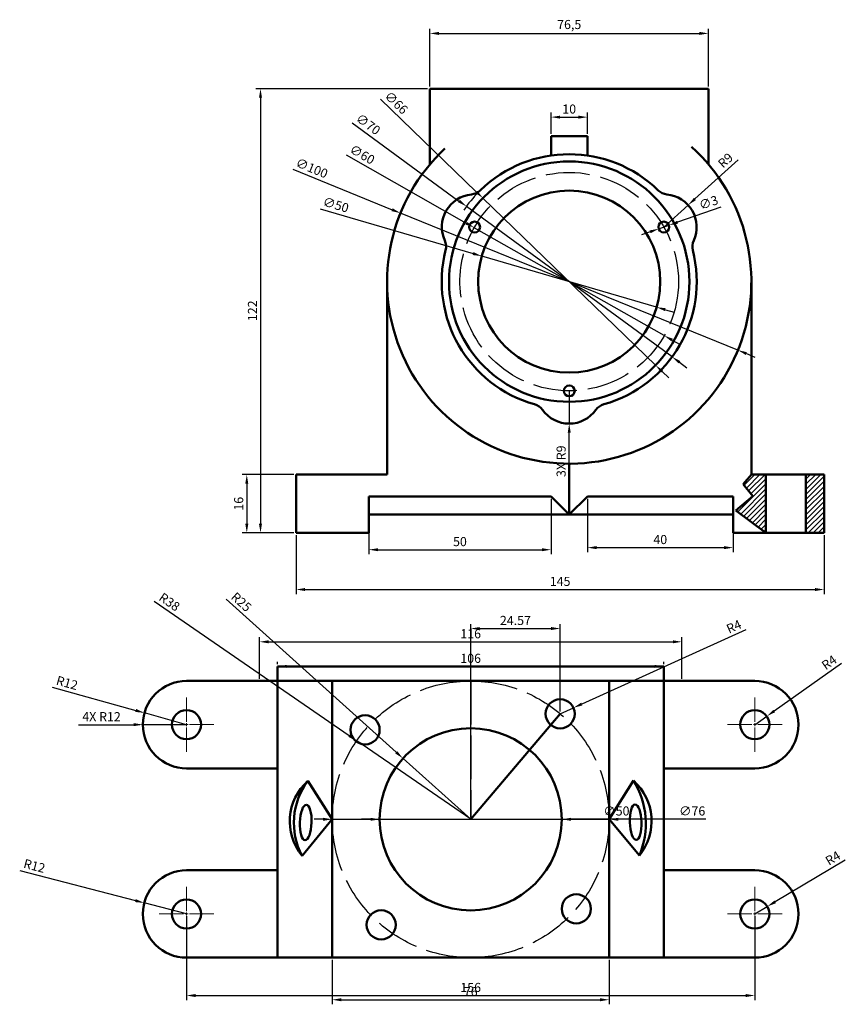
# Model space of a CAD drawing. Units: millimetres. Extents: x 1140 to 1880, y 1480 to 1815.
# Tile 1 of 3: x 1140 to 1366, y 1537 to 1807. Entities that reach past the tile are written whole.
import ezdxf

# ---------------------------------------------------------------- set-up
doc = ezdxf.new("R2010")
doc.units = ezdxf.units.MM
doc.linetypes.add('ACAD_ISO02W100', pattern=[15, 12, -3])
doc.linetypes.add('CENTER2', pattern=[28.575, 19.05, -3.175, 3.175, -3.175])
for name, color, linetype, lineweight in [('M-CNTR', 1, 'CENTER2', 18), ('M-DIMS', 2, 'Continuous', 25), ('M-HATC', 8, 'Continuous', 18), ('M-HIDN', 6, 'ACAD_ISO02W100', 25), ('M-OUTL', 7, 'Continuous', 50)]:
    doc.layers.add(name, color=color, linetype=linetype, lineweight=lineweight)
doc.styles.get("Standard").update_dxf_attribs({"font": 'arial.ttf'})
doc.dimstyles.new('ISO-25', dxfattribs={"dimtxt": 2.5, "dimasz": 2.5, "dimexe": 1.25, "dimexo": 0.625, "dimtad": 1, "dimtxsty": 'Standard', "dimcen": 2.5, "dimadec": 0, "dimazin": 0, "dimtfac": 1, "dimtmove": 0, "dimatfit": 3, "dimfxl": 1, "dimarcsym": 0})

# ---------------------------------------------------------------- blocks, each defined once
blk = doc.blocks.new('*U1')
blk.add_circle((0, 0), 1.5)
blk = doc.blocks.new('*U2')
at = {"layer": 'M-OUTL', "color": 0, "linetype": 'ByBlock', "lineweight": -2, "transparency": 16777216}
for p, rotation in [((1264.48, 1750.45), 240), ((1316.44, 1750.45), 119.9999999999999)]:
    blk.add_blockref('*U1', p, dxfattribs=dict(at, rotation=rotation))
blk.add_blockref('*U1', (1290.46, 1705.45), dxfattribs=at)
blk = doc.blocks.new('*U3')
at = {"layer": 'M-CNTR', "color": 0, "transparency": 16777216}
for p, q in [((0, 0.8), (0, 7.5)), ((-7.5, 0), (-0.8, 0)), ((0.8, 0), (7.5, 0)), ((0, -7.5), (0, -0.8))]:
    blk.add_line(p, q, dxfattribs=at)
at = {"layer": 'M-CNTR', "color": 0, "linetype": 'Continuous', "transparency": 16777216}
for p, q in [((-0.4, 0), (0.4, 0)), ((0, -0.4), (0, 0.4))]:
    blk.add_line(p, q, dxfattribs=at)
blk = doc.blocks.new('*U4')
at = {"layer": 'M-CNTR', "color": 0, "transparency": 16777216}
for p, q in [((0, 0.8), (0, 7.5)), ((-7.5, 0), (-0.8, 0)), ((0.8, 0), (7.5, 0)), ((0, -7.5), (0, -0.8))]:
    blk.add_line(p, q, dxfattribs=at)
at = {"layer": 'M-CNTR', "color": 0, "linetype": 'Continuous', "transparency": 16777216}
for p, q in [((-0.4, 0), (0.4, 0)), ((0, -0.4), (0, 0.4))]:
    blk.add_line(p, q, dxfattribs=at)
blk = doc.blocks.new('*U5')
at = {"layer": 'M-CNTR', "color": 0, "transparency": 16777216}
for p, q in [((0, 0.8), (0, 7.5)), ((-7.5, 0), (-0.8, 0)), ((0.8, 0), (7.5, 0)), ((0, -7.5), (0, -0.8))]:
    blk.add_line(p, q, dxfattribs=at)
at = {"layer": 'M-CNTR', "color": 0, "linetype": 'Continuous', "transparency": 16777216}
for p, q in [((-0.4, 0), (0.4, 0)), ((0, -0.4), (0, 0.4))]:
    blk.add_line(p, q, dxfattribs=at)
blk = doc.blocks.new('*U6')
at = {"layer": 'M-CNTR', "color": 0, "transparency": 16777216}
for p, q in [((0, 0.8), (0, 7.5)), ((-7.5, 0), (-0.8, 0)), ((0.8, 0), (7.5, 0)), ((0, -7.5), (0, -0.8))]:
    blk.add_line(p, q, dxfattribs=at)
at = {"layer": 'M-CNTR', "color": 0, "linetype": 'Continuous', "transparency": 16777216}
for p, q in [((-0.4, 0), (0.4, 0)), ((0, -0.4), (0, 0.4))]:
    blk.add_line(p, q, dxfattribs=at)
blk = doc.blocks.new('*U7')
blk.add_circle((0, 0), 4)
blk = doc.blocks.new('*U8')
at = {"layer": 'M-OUTL', "color": 0, "linetype": 'ByBlock', "lineweight": -2, "transparency": 16777216}
blk.add_blockref('*U7', (1287.98, 1616.75), dxfattribs=at)
for p, rotation in [((1234.42, 1612.33), 90.00000000000003), ((1292.4, 1563.19), 269.9999999999999), ((1238.84, 1558.77), 180)]:
    blk.add_blockref('*U7', p, dxfattribs=dict(at, rotation=rotation))
blk = doc.blocks.new('*D9')
at = {"layer": 'Defpoints', "color": 0, "transparency": 16777216}
for p in [(1328.71, 1803.63), (1252.21, 1788.45), (1328.71, 1788.45)]:
    blk.add_point(p, dxfattribs=at)
at = {"layer": 'M-DIMS', "color": 0, "lineweight": -2, "transparency": 16777216}
for p, q in [((1252.21, 1789.08), (1252.21, 1804.88)), ((1328.71, 1789.08), (1328.71, 1804.88)), ((1254.71, 1803.63), (1326.21, 1803.63))]:
    blk.add_line(p, q, dxfattribs=at)
at = {"layer": 'M-DIMS', "color": 0, "transparency": 16777216}
for points in [[(1254.71, 1804.05), (1254.71, 1803.22), (1252.21, 1803.63)], [(1326.21, 1804.05), (1326.21, 1803.22), (1328.71, 1803.63)]]:
    blk.add_solid(points, dxfattribs=at)
at = {"layer": 'M-DIMS', "color": 0, "transparency": 16777216, "insert": (1290.46, 1805.76), "char_height": 2.5, "attachment_point": 5}
blk.add_mtext('76,5', dxfattribs=at)
blk = doc.blocks.new('*D10')
at = {"layer": 'Defpoints', "color": 0, "transparency": 16777216}
for p in [(1215.46, 1666.45), (1360.46, 1666.45), (1360.46, 1650.88)]:
    blk.add_point(p, dxfattribs=at)
at = {"layer": 'M-DIMS', "color": 0, "lineweight": -2, "transparency": 16777216}
for p, q in [((1215.46, 1665.83), (1215.46, 1649.63)), ((1360.46, 1665.83), (1360.46, 1649.63)), ((1217.96, 1650.88), (1357.96, 1650.88))]:
    blk.add_line(p, q, dxfattribs=at)
at = {"layer": 'M-DIMS', "color": 0, "transparency": 16777216}
for points in [[(1217.96, 1651.3), (1217.96, 1650.47), (1215.46, 1650.88)], [(1357.96, 1651.3), (1357.96, 1650.47), (1360.46, 1650.88)]]:
    blk.add_solid(points, dxfattribs=at)
at = {"layer": 'M-DIMS', "color": 0, "transparency": 16777216, "insert": (1287.96, 1652.79), "char_height": 2.5, "attachment_point": 5}
blk.add_mtext('145', dxfattribs=at)
blk = doc.blocks.new('*D11')
at = {"layer": 'Defpoints', "color": 0, "transparency": 16777216}
for p in [(1215.46, 1682.45), (1201.94, 1666.45), (1215.46, 1666.45)]:
    blk.add_point(p, dxfattribs=at)
at = {"layer": 'M-DIMS', "color": 0, "lineweight": -2, "transparency": 16777216}
for p, q in [((1214.83, 1682.45), (1200.69, 1682.45)), ((1201.94, 1679.95), (1201.94, 1668.95)), ((1214.83, 1666.45), (1200.69, 1666.45))]:
    blk.add_line(p, q, dxfattribs=at)
at = {"layer": 'M-DIMS', "color": 0, "transparency": 16777216}
for points in [[(1201.53, 1679.95), (1202.36, 1679.95), (1201.94, 1682.45)], [(1201.53, 1668.95), (1202.36, 1668.95), (1201.94, 1666.45)]]:
    blk.add_solid(points, dxfattribs=at)
at = {"layer": 'M-DIMS', "color": 0, "transparency": 16777216, "insert": (1200.04, 1674.45), "char_height": 2.5, "attachment_point": 5, "rotation": 90}
blk.add_mtext('16', dxfattribs=at)
blk = doc.blocks.new('*D12')
at = {"layer": 'Defpoints', "color": 0, "transparency": 16777216}
for p in [(1235.46, 1676.45), (1285.46, 1676.45), (1285.46, 1661.82)]:
    blk.add_point(p, dxfattribs=at)
at = {"layer": 'M-DIMS', "color": 0, "lineweight": -2, "transparency": 16777216}
for p, q in [((1235.46, 1675.83), (1235.46, 1660.57)), ((1285.46, 1675.83), (1285.46, 1660.57)), ((1237.96, 1661.82), (1282.96, 1661.82))]:
    blk.add_line(p, q, dxfattribs=at)
at = {"layer": 'M-DIMS', "color": 0, "transparency": 16777216}
for points in [[(1237.96, 1662.23), (1237.96, 1661.4), (1235.46, 1661.82)], [(1282.96, 1662.23), (1282.96, 1661.4), (1285.46, 1661.82)]]:
    blk.add_solid(points, dxfattribs=at)
at = {"layer": 'M-DIMS', "color": 0, "transparency": 16777216, "insert": (1260.46, 1663.72), "char_height": 2.5, "attachment_point": 5}
blk.add_mtext('50', dxfattribs=at)
blk = doc.blocks.new('*D13')
at = {"layer": 'Defpoints', "color": 0, "transparency": 16777216}
for p in [(1295.46, 1676.45), (1335.46, 1676.45), (1335.46, 1662.39)]:
    blk.add_point(p, dxfattribs=at)
at = {"layer": 'M-DIMS', "color": 0, "lineweight": -2, "transparency": 16777216}
for p, q in [((1295.46, 1675.83), (1295.46, 1661.14)), ((1335.46, 1675.83), (1335.46, 1661.14)), ((1297.96, 1662.39), (1332.96, 1662.39))]:
    blk.add_line(p, q, dxfattribs=at)
at = {"layer": 'M-DIMS', "color": 0, "transparency": 16777216}
for points in [[(1297.96, 1662.81), (1297.96, 1661.97), (1295.46, 1662.39)], [(1332.96, 1662.81), (1332.96, 1661.97), (1335.46, 1662.39)]]:
    blk.add_solid(points, dxfattribs=at)
at = {"layer": 'M-DIMS', "color": 0, "transparency": 16777216, "insert": (1315.46, 1664.29), "char_height": 2.5, "attachment_point": 5}
blk.add_mtext('40', dxfattribs=at)
blk = doc.blocks.new('*D14')
at = {"layer": 'Defpoints', "color": 0, "transparency": 16777216}
for p in [(1244.14, 1754.27), (1336.78, 1716.63)]:
    blk.add_point(p, dxfattribs=at)
at = {"layer": 'M-DIMS', "color": 0, "lineweight": -2, "transparency": 16777216}
for p, q in [((1214.54, 1766.3), (1241.82, 1755.21)), ((1336.78, 1716.63), (1244.14, 1754.27)), ((1339.1, 1715.69), (1341.41, 1714.75))]:
    blk.add_line(p, q, dxfattribs=at)
at = {"layer": 'M-DIMS', "color": 0, "transparency": 16777216}
for points in [[(1241.98, 1755.6), (1241.66, 1754.83), (1244.14, 1754.27)], [(1339.25, 1716.07), (1338.94, 1715.3), (1336.78, 1716.63)]]:
    blk.add_solid(points, dxfattribs=at)
at = {"layer": 'M-DIMS', "color": 0, "transparency": 16777216, "insert": (1219.67, 1766.34), "char_height": 2.5, "attachment_point": 5, "rotation": 337.8882}
blk.add_mtext('∅100', dxfattribs=at)
blk = doc.blocks.new('*D15')
at = {"layer": 'Defpoints', "color": 0, "transparency": 16777216}
for p in [(1262.22, 1756.13), (1318.7, 1714.77)]:
    blk.add_point(p, dxfattribs=at)
at = {"layer": 'M-DIMS', "color": 0, "lineweight": -2, "transparency": 16777216}
for p, q in [((1230.88, 1779.07), (1260.2, 1757.6)), ((1318.7, 1714.77), (1262.22, 1756.13)), ((1320.72, 1713.3), (1322.73, 1711.82))]:
    blk.add_line(p, q, dxfattribs=at)
blk.add_arc((1290.46, 1735.45), 35, 135.26, 145.8359, dxfattribs=at)
at = {"layer": 'M-DIMS', "color": 0, "transparency": 16777216}
for points in [[(1260.45, 1757.94), (1259.95, 1757.27), (1262.22, 1756.13)], [(1320.96, 1713.63), (1320.47, 1712.96), (1318.7, 1714.77)]]:
    blk.add_solid(points, dxfattribs=at)
at = {"layer": 'M-DIMS', "color": 0, "transparency": 16777216, "insert": (1235.09, 1778.43), "char_height": 2.5, "attachment_point": 5, "rotation": 323.7896}
blk.add_mtext('∅70', dxfattribs=at)
blk = doc.blocks.new('*D16')
at = {"layer": 'Defpoints', "color": 0, "transparency": 16777216}
for p in [(1266.75, 1758.4), (1314.17, 1712.5)]:
    blk.add_point(p, dxfattribs=at)
at = {"layer": 'M-DIMS', "color": 0, "lineweight": -2, "transparency": 16777216}
for p, q in [((1238.68, 1785.58), (1264.95, 1760.14)), ((1314.17, 1712.5), (1266.75, 1758.4)), ((1315.96, 1710.76), (1317.76, 1709.02))]:
    blk.add_line(p, q, dxfattribs=at)
at = {"layer": 'M-DIMS', "color": 0, "transparency": 16777216}
for points in [[(1265.24, 1760.44), (1264.66, 1759.84), (1266.75, 1758.4)], [(1316.25, 1711.06), (1315.67, 1710.46), (1314.17, 1712.5)]]:
    blk.add_solid(points, dxfattribs=at)
at = {"layer": 'M-DIMS', "color": 0, "transparency": 16777216, "insert": (1242.76, 1784.37), "char_height": 2.5, "attachment_point": 5, "rotation": 315.9271}
blk.add_mtext('∅66', dxfattribs=at)
blk = doc.blocks.new('*D17')
at = {"layer": 'Defpoints', "color": 0, "transparency": 16777216}
for p in [(1264.38, 1750.27), (1316.54, 1720.63)]:
    blk.add_point(p, dxfattribs=at)
at = {"layer": 'M-DIMS', "color": 0, "lineweight": -2, "transparency": 16777216}
for p, q in [((1229.22, 1770.25), (1262.2, 1751.51)), ((1316.54, 1720.63), (1264.38, 1750.27)), ((1318.71, 1719.39), (1320.89, 1718.16))]:
    blk.add_line(p, q, dxfattribs=at)
at = {"layer": 'M-DIMS', "color": 0, "transparency": 16777216}
for points in [[(1262.41, 1751.87), (1262, 1751.15), (1264.38, 1750.27)], [(1318.92, 1719.75), (1318.51, 1719.03), (1316.54, 1720.63)]]:
    blk.add_solid(points, dxfattribs=at)
at = {"layer": 'M-DIMS', "color": 0, "transparency": 16777216, "insert": (1233.48, 1770.1), "char_height": 2.5, "attachment_point": 5, "rotation": 330.3907}
blk.add_mtext('∅60', dxfattribs=at)
blk = doc.blocks.new('*D18')
at = {"layer": 'Defpoints', "color": 0, "transparency": 16777216}
for p in [(1266.46, 1742.46), (1314.45, 1728.44)]:
    blk.add_point(p, dxfattribs=at)
at = {"layer": 'M-DIMS', "color": 0, "lineweight": -2, "transparency": 16777216}
for p, q in [((1222.12, 1755.42), (1264.06, 1743.16)), ((1314.45, 1728.44), (1266.46, 1742.46)), ((1316.85, 1727.74), (1319.25, 1727.04))]:
    blk.add_line(p, q, dxfattribs=at)
at = {"layer": 'M-DIMS', "color": 0, "transparency": 16777216}
for points in [[(1264.18, 1743.56), (1263.94, 1742.76), (1266.46, 1742.46)], [(1316.97, 1728.14), (1316.74, 1727.34), (1314.45, 1728.44)]]:
    blk.add_solid(points, dxfattribs=at)
at = {"layer": 'M-DIMS', "color": 0, "transparency": 16777216, "insert": (1226.3, 1756.25), "char_height": 2.5, "attachment_point": 5, "rotation": 343.7126}
blk.add_mtext('∅50', dxfattribs=at)
blk = doc.blocks.new('*D19')
at = {"layer": 'Defpoints', "color": 0, "transparency": 16777216}
for p in [(1323.11, 1756.49), (1316.44, 1750.45)]:
    blk.add_point(p, dxfattribs=at)
at = {"layer": 'M-DIMS', "color": 0, "lineweight": -2, "transparency": 16777216}
for p, q in [((1336.81, 1768.88), (1324.97, 1758.16)), ((1316.44, 1750.45), (1323.11, 1756.49))]:
    blk.add_line(p, q, dxfattribs=at)
at = {"layer": 'M-DIMS', "color": 0, "transparency": 16777216}
blk.add_solid([(1324.69, 1758.47), (1325.25, 1757.86), (1323.11, 1756.49)], dxfattribs=at)
at = {"layer": 'M-DIMS', "color": 0, "transparency": 16777216, "insert": (1333.57, 1768.51), "char_height": 2.5, "attachment_point": 5, "rotation": 42.1321}
blk.add_mtext('R9', dxfattribs=at)
blk = doc.blocks.new('*D20')
at = {"layer": 'Defpoints', "color": 0, "transparency": 16777216}
for p in [(1315.02, 1749.96), (1317.85, 1750.94)]:
    blk.add_point(p, dxfattribs=at)
at = {"layer": 'M-DIMS', "color": 0, "lineweight": -2, "transparency": 16777216}
for p, q in [((1332.11, 1755.93), (1320.22, 1751.77)), ((1315.02, 1749.96), (1317.85, 1750.94)), ((1312.66, 1749.13), (1310.3, 1748.31))]:
    blk.add_line(p, q, dxfattribs=at)
at = {"layer": 'M-DIMS', "color": 0, "transparency": 16777216}
for points in [[(1312.53, 1749.52), (1312.8, 1748.74), (1315.02, 1749.96)], [(1320.08, 1752.16), (1320.35, 1751.38), (1317.85, 1750.94)]]:
    blk.add_solid(points, dxfattribs=at)
at = {"layer": 'M-DIMS', "color": 0, "transparency": 16777216, "insert": (1328.81, 1756.86), "char_height": 2.5, "attachment_point": 5, "rotation": 19.2549}
blk.add_mtext('∅3', dxfattribs=at)
blk = doc.blocks.new('*D21')
at = {"layer": 'Defpoints', "color": 0, "transparency": 16777216}
for p in [(1295.46, 1780.64), (1285.46, 1775.45), (1295.46, 1775.45)]:
    blk.add_point(p, dxfattribs=at)
at = {"layer": 'M-DIMS', "color": 0, "lineweight": -2, "transparency": 16777216}
for p, q in [((1285.46, 1776.08), (1285.46, 1781.89)), ((1287.96, 1780.64), (1292.96, 1780.64)), ((1295.46, 1776.08), (1295.46, 1781.89))]:
    blk.add_line(p, q, dxfattribs=at)
at = {"layer": 'M-DIMS', "color": 0, "transparency": 16777216}
for points in [[(1287.96, 1781.05), (1287.96, 1780.22), (1285.46, 1780.64)], [(1292.96, 1781.05), (1292.96, 1780.22), (1295.46, 1780.64)]]:
    blk.add_solid(points, dxfattribs=at)
at = {"layer": 'M-DIMS', "color": 0, "transparency": 16777216, "insert": (1290.46, 1782.54), "char_height": 2.5, "attachment_point": 5}
blk.add_mtext('10', dxfattribs=at)
blk = doc.blocks.new('*D22')
at = {"layer": 'Defpoints', "color": 0, "transparency": 16777216}
for p in [(1210.41, 1629.76), (1316.41, 1629.76), (1316.41, 1629.76)]:
    blk.add_point(p, dxfattribs=at)
at = {"layer": 'M-DIMS', "color": 0, "lineweight": -2, "transparency": 16777216}
for p, q in [((1210.41, 1630.39), (1210.41, 1631.01)), ((1316.41, 1630.39), (1316.41, 1631.01)), ((1212.91, 1629.76), (1313.91, 1629.76))]:
    blk.add_line(p, q, dxfattribs=at)
at = {"layer": 'M-DIMS', "color": 0, "transparency": 16777216}
for points in [[(1212.91, 1630.18), (1212.91, 1629.35), (1210.41, 1629.76)], [(1313.91, 1630.18), (1313.91, 1629.35), (1316.41, 1629.76)]]:
    blk.add_solid(points, dxfattribs=at)
at = {"layer": 'M-DIMS', "color": 0, "transparency": 16777216, "insert": (1263.41, 1631.66), "char_height": 2.5, "attachment_point": 5}
blk.add_mtext('106', dxfattribs=at)
blk = doc.blocks.new('*D23')
at = {"layer": 'Defpoints', "color": 0, "transparency": 16777216}
for p in [(1321.41, 1636.52), (1205.41, 1625.76), (1321.41, 1625.76)]:
    blk.add_point(p, dxfattribs=at)
at = {"layer": 'M-DIMS', "color": 0, "lineweight": -2, "transparency": 16777216}
for p, q in [((1205.41, 1626.39), (1205.41, 1637.77)), ((1207.91, 1636.52), (1318.91, 1636.52)), ((1321.41, 1626.39), (1321.41, 1637.77))]:
    blk.add_line(p, q, dxfattribs=at)
at = {"layer": 'M-DIMS', "color": 0, "transparency": 16777216}
for points in [[(1207.91, 1636.94), (1207.91, 1636.11), (1205.41, 1636.52)], [(1318.91, 1636.94), (1318.91, 1636.11), (1321.41, 1636.52)]]:
    blk.add_solid(points, dxfattribs=at)
at = {"layer": 'M-DIMS', "color": 0, "transparency": 16777216, "insert": (1263.41, 1638.42), "char_height": 2.5, "attachment_point": 5}
blk.add_mtext('116', dxfattribs=at)
blk = doc.blocks.new('*D24')
at = {"layer": 'Defpoints', "color": 0, "transparency": 16777216}
for p in [(1225.41, 1549.76), (1301.41, 1549.76), (1301.41, 1538.2)]:
    blk.add_point(p, dxfattribs=at)
at = {"layer": 'M-DIMS', "color": 0, "lineweight": -2, "transparency": 16777216}
for p, q in [((1225.41, 1549.14), (1225.41, 1536.95)), ((1301.41, 1549.14), (1301.41, 1536.95)), ((1227.91, 1538.2), (1298.91, 1538.2))]:
    blk.add_line(p, q, dxfattribs=at)
at = {"layer": 'M-DIMS', "color": 0, "transparency": 16777216}
for points in [[(1227.91, 1538.62), (1227.91, 1537.78), (1225.41, 1538.2)], [(1298.91, 1538.62), (1298.91, 1537.78), (1301.41, 1538.2)]]:
    blk.add_solid(points, dxfattribs=at)
at = {"layer": 'M-DIMS', "color": 0, "transparency": 16777216, "insert": (1263.41, 1540.1), "char_height": 2.5, "attachment_point": 5}
blk.add_mtext('76', dxfattribs=at)
blk = doc.blocks.new('*D25')
at = {"layer": 'Defpoints', "color": 0, "transparency": 16777216}
for p in [(1173.85, 1617), (1185.41, 1613.76)]:
    blk.add_point(p, dxfattribs=at)
at = {"layer": 'M-DIMS', "color": 0, "lineweight": -2, "transparency": 16777216}
for p, q in [((1148.55, 1624.08), (1171.44, 1617.67)), ((1185.41, 1613.76), (1173.85, 1617))]:
    blk.add_line(p, q, dxfattribs=at)
at = {"layer": 'M-DIMS', "color": 0, "transparency": 16777216}
blk.add_solid([(1171.56, 1618.07), (1171.33, 1617.27), (1173.85, 1617)], dxfattribs=at)
at = {"layer": 'M-DIMS', "color": 0, "transparency": 16777216, "insert": (1152.52, 1624.92), "char_height": 2.5, "attachment_point": 5, "rotation": 344.3673}
blk.add_mtext('R12', dxfattribs=at)
blk = doc.blocks.new('*D26')
at = {"layer": 'Defpoints', "color": 0, "transparency": 16777216}
for p in [(1173.8, 1564.8), (1185.41, 1561.76)]:
    blk.add_point(p, dxfattribs=at)
at = {"layer": 'M-DIMS', "color": 0, "lineweight": -2, "transparency": 16777216}
for p, q in [((1139.6, 1573.75), (1171.38, 1565.43)), ((1185.41, 1561.76), (1173.8, 1564.8))]:
    blk.add_line(p, q, dxfattribs=at)
at = {"layer": 'M-DIMS', "color": 0, "transparency": 16777216}
blk.add_solid([(1171.48, 1565.84), (1171.27, 1565.03), (1173.8, 1564.8)], dxfattribs=at)
at = {"layer": 'M-DIMS', "color": 0, "transparency": 16777216, "insert": (1143.56, 1574.66), "char_height": 2.5, "attachment_point": 5, "rotation": 345.3361}
blk.add_mtext('R12', dxfattribs=at)
blk = doc.blocks.new('*D27')
at = {"layer": 'Defpoints', "color": 0, "transparency": 16777216}
for p in [(1344.68, 1616.07), (1341.41, 1613.76)]:
    blk.add_point(p, dxfattribs=at)
at = {"layer": 'M-DIMS', "color": 0, "lineweight": -2, "transparency": 16777216}
for p, q in [((1365.25, 1630.57), (1346.72, 1617.51)), ((1341.41, 1613.76), (1344.68, 1616.07))]:
    blk.add_line(p, q, dxfattribs=at)
at = {"layer": 'M-DIMS', "color": 0, "transparency": 16777216}
blk.add_solid([(1346.48, 1617.85), (1346.96, 1617.17), (1344.68, 1616.07)], dxfattribs=at)
at = {"layer": 'M-DIMS', "color": 0, "transparency": 16777216, "insert": (1362.01, 1630.59), "char_height": 2.5, "attachment_point": 5, "rotation": 35.1929}
blk.add_mtext('R4', dxfattribs=at)
blk = doc.blocks.new('*D28')
at = {"layer": 'Defpoints', "color": 0, "transparency": 16777216}
for p in [(1344.84, 1563.81), (1341.41, 1561.76)]:
    blk.add_point(p, dxfattribs=at)
at = {"layer": 'M-DIMS', "color": 0, "lineweight": -2, "transparency": 16777216}
for p, q in [((1366.25, 1576.57), (1346.99, 1565.09)), ((1341.41, 1561.76), (1344.84, 1563.81))]:
    blk.add_line(p, q, dxfattribs=at)
at = {"layer": 'M-DIMS', "color": 0, "transparency": 16777216}
blk.add_solid([(1346.78, 1565.45), (1347.2, 1564.73), (1344.84, 1563.81)], dxfattribs=at)
at = {"layer": 'M-DIMS', "color": 0, "transparency": 16777216, "insert": (1363.02, 1576.83), "char_height": 2.5, "attachment_point": 5, "rotation": 30.7913}
blk.add_mtext('R4', dxfattribs=at)
blk = doc.blocks.new('*D29')
at = {"layer": 'Defpoints', "color": 0, "transparency": 16777216}
for p in [(1232.12, 1609.33), (1263.41, 1587.76)]:
    blk.add_point(p, dxfattribs=at)
at = {"layer": 'M-DIMS', "color": 0, "lineweight": -2, "transparency": 16777216}
for p, q in [((1176.48, 1647.68), (1230.06, 1610.75)), ((1263.41, 1587.76), (1232.12, 1609.33))]:
    blk.add_line(p, q, dxfattribs=at)
at = {"layer": 'M-DIMS', "color": 0, "transparency": 16777216}
blk.add_solid([(1230.3, 1611.09), (1229.83, 1610.41), (1232.12, 1609.33)], dxfattribs=at)
at = {"layer": 'M-DIMS', "color": 0, "transparency": 16777216, "insert": (1180.54, 1647.2), "char_height": 2.5, "attachment_point": 5, "rotation": 325.4215}
blk.add_mtext('R38', dxfattribs=at)
blk = doc.blocks.new('*D30')
at = {"layer": 'Defpoints', "color": 0, "transparency": 16777216}
for p in [(1244.83, 1604.49), (1263.41, 1587.76)]:
    blk.add_point(p, dxfattribs=at)
at = {"layer": 'M-DIMS', "color": 0, "lineweight": -2, "transparency": 16777216}
for p, q in [((1196.27, 1648.24), (1242.97, 1606.17)), ((1263.41, 1587.76), (1244.83, 1604.49))]:
    blk.add_line(p, q, dxfattribs=at)
at = {"layer": 'M-DIMS', "color": 0, "transparency": 16777216}
blk.add_solid([(1243.25, 1606.48), (1242.7, 1605.86), (1244.83, 1604.49)], dxfattribs=at)
at = {"layer": 'M-DIMS', "color": 0, "transparency": 16777216, "insert": (1200.23, 1647.23), "char_height": 2.5, "attachment_point": 5, "rotation": 317.989}
blk.add_mtext('R25', dxfattribs=at)
blk = doc.blocks.new('*D31')
at = {"layer": 'Defpoints', "color": 0, "transparency": 16777216}
for p in [(1291.62, 1618.4), (1287.98, 1616.75)]:
    blk.add_point(p, dxfattribs=at)
at = {"layer": 'M-DIMS', "color": 0, "lineweight": -2, "transparency": 16777216}
for p, q in [((1338.98, 1639.78), (1293.9, 1619.43)), ((1287.98, 1616.75), (1291.62, 1618.4))]:
    blk.add_line(p, q, dxfattribs=at)
at = {"layer": 'M-DIMS', "color": 0, "transparency": 16777216}
blk.add_solid([(1293.73, 1619.81), (1294.07, 1619.05), (1291.62, 1618.4)], dxfattribs=at)
at = {"layer": 'M-DIMS', "color": 0, "transparency": 16777216, "insert": (1335.8, 1640.41), "char_height": 2.5, "attachment_point": 5, "rotation": 24.3041}
blk.add_mtext('R4', dxfattribs=at)
blk = doc.blocks.new('HOLE-D8')
blk.add_circle((4, 4), 4)
blk = doc.blocks.new('*D83')
at = {"layer": 'Defpoints', "color": 0, "transparency": 16777216}
for p in [(1252.21, 1788.45), (1205.71, 1666.45), (1215.46, 1666.45)]:
    blk.add_point(p, dxfattribs=at)
at = {"layer": 'M-DIMS', "color": 0, "lineweight": -2, "transparency": 16777216}
for p, q in [((1251.58, 1788.45), (1204.46, 1788.45)), ((1205.71, 1785.95), (1205.71, 1668.95)), ((1214.83, 1666.45), (1204.46, 1666.45))]:
    blk.add_line(p, q, dxfattribs=at)
at = {"layer": 'M-DIMS', "color": 0, "transparency": 16777216}
for points in [[(1205.29, 1785.95), (1206.12, 1785.95), (1205.71, 1788.45)], [(1205.29, 1668.95), (1206.12, 1668.95), (1205.71, 1666.45)]]:
    blk.add_solid(points, dxfattribs=at)
at = {"layer": 'M-DIMS', "color": 0, "transparency": 16777216, "insert": (1203.83, 1727.45), "char_height": 2.5, "attachment_point": 5, "rotation": 90}
blk.add_mtext('122', dxfattribs=at)
blk = doc.blocks.new('*D84')
at = {"layer": 'Defpoints', "color": 0, "transparency": 16777216}
for p in [(1185.41, 1561.76), (1341.41, 1561.76), (1341.41, 1539.36)]:
    blk.add_point(p, dxfattribs=at)
at = {"layer": 'M-DIMS', "color": 0, "lineweight": -2, "transparency": 16777216}
for p, q in [((1185.41, 1561.14), (1185.41, 1538.11)), ((1341.41, 1561.14), (1341.41, 1538.11)), ((1187.91, 1539.36), (1338.91, 1539.36))]:
    blk.add_line(p, q, dxfattribs=at)
at = {"layer": 'M-DIMS', "color": 0, "transparency": 16777216}
for points in [[(1187.91, 1539.78), (1187.91, 1538.95), (1185.41, 1539.36)], [(1338.91, 1539.78), (1338.91, 1538.95), (1341.41, 1539.36)]]:
    blk.add_solid(points, dxfattribs=at)
at = {"layer": 'M-DIMS', "color": 0, "transparency": 16777216, "insert": (1263.41, 1541.26), "char_height": 2.5, "attachment_point": 5}
blk.add_mtext('156', dxfattribs=at)
blk = doc.blocks.new('*D85')
at = {"layer": 'Defpoints', "color": 0, "transparency": 16777216}
for p in [(1287.98, 1640.16), (1287.98, 1616.75), (1263.41, 1587.76)]:
    blk.add_point(p, dxfattribs=at)
at = {"layer": 'M-DIMS', "color": 0, "lineweight": -2, "transparency": 16777216}
for p, q in [((1263.41, 1588.39), (1263.41, 1641.41)), ((1265.91, 1640.16), (1285.48, 1640.16)), ((1287.98, 1617.38), (1287.98, 1641.41))]:
    blk.add_line(p, q, dxfattribs=at)
at = {"layer": 'M-DIMS', "color": 0, "transparency": 16777216}
for points in [[(1265.91, 1640.58), (1265.91, 1639.75), (1263.41, 1640.16)], [(1285.48, 1640.58), (1285.48, 1639.75), (1287.98, 1640.16)]]:
    blk.add_solid(points, dxfattribs=at)
at = {"layer": 'M-DIMS', "color": 0, "transparency": 16777216, "insert": (1275.69, 1642.06), "char_height": 2.5, "attachment_point": 5}
blk.add_mtext('24.57', dxfattribs=at)
blk = doc.blocks.new('*D94')
at = {"layer": 'Defpoints', "color": 0, "transparency": 16777216}
for p in [(1290.46, 1705.45), (1290.46, 1696.45)]:
    blk.add_point(p, dxfattribs=at)
at = {"layer": 'M-DIMS', "color": 0, "lineweight": -2, "transparency": 16777216}
for p, q in [((1290.46, 1705.45), (1290.46, 1696.45)), ((1290.46, 1680.79), (1290.46, 1693.95))]:
    blk.add_line(p, q, dxfattribs=at)
at = {"layer": 'M-DIMS', "color": 0, "transparency": 16777216}
blk.add_solid([(1290.04, 1693.95), (1290.87, 1693.95), (1290.46, 1696.45)], dxfattribs=at)
at = {"layer": 'M-DIMS', "color": 0, "transparency": 16777216, "insert": (1288.56, 1686.12), "char_height": 2.5, "attachment_point": 5, "rotation": 89.9994}
blk.add_mtext('3X R9', dxfattribs=at)
blk = doc.blocks.new('*D95')
at = {"layer": 'Defpoints', "color": 0, "transparency": 16777216}
for p in [(1225.41, 1587.76), (1301.41, 1587.76)]:
    blk.add_point(p, dxfattribs=at)
at = {"layer": 'M-DIMS', "color": 0, "lineweight": -2, "transparency": 16777216}
for p, q in [((1222.91, 1587.76), (1220.41, 1587.76)), ((1225.41, 1587.76), (1301.41, 1587.76)), ((1327.98, 1587.76), (1303.91, 1587.76))]:
    blk.add_line(p, q, dxfattribs=at)
at = {"layer": 'M-DIMS', "color": 0, "transparency": 16777216}
for points in [[(1222.91, 1588.18), (1222.91, 1587.35), (1225.41, 1587.76)], [(1303.91, 1588.18), (1303.91, 1587.35), (1301.41, 1587.76)]]:
    blk.add_solid(points, dxfattribs=at)
at = {"layer": 'M-DIMS', "color": 0, "transparency": 16777216, "insert": (1324.21, 1589.73), "char_height": 2.5, "attachment_point": 5, "rotation": 0}
blk.add_mtext('∅76', dxfattribs=at)
blk = doc.blocks.new('*D96')
at = {"layer": 'Defpoints', "color": 0, "transparency": 16777216}
for p in [(1238.41, 1587.76), (1288.41, 1587.76)]:
    blk.add_point(p, dxfattribs=at)
at = {"layer": 'M-DIMS', "color": 0, "lineweight": -2, "transparency": 16777216}
for p, q in [((1235.91, 1587.76), (1233.41, 1587.76)), ((1238.41, 1587.76), (1288.41, 1587.76)), ((1307.18, 1587.76), (1290.91, 1587.76))]:
    blk.add_line(p, q, dxfattribs=at)
at = {"layer": 'M-DIMS', "color": 0, "transparency": 16777216}
for points in [[(1235.91, 1588.18), (1235.91, 1587.35), (1238.41, 1587.76)], [(1290.91, 1588.18), (1290.91, 1587.35), (1288.41, 1587.76)]]:
    blk.add_solid(points, dxfattribs=at)
at = {"layer": 'M-DIMS', "color": 0, "transparency": 16777216, "insert": (1303.41, 1589.73), "char_height": 2.5, "attachment_point": 5, "rotation": 0}
blk.add_mtext('∅50', dxfattribs=at)
blk = doc.blocks.new('*D97')
at = {"layer": 'Defpoints', "color": 0, "transparency": 16777216}
for p in [(1173.41, 1613.76), (1185.41, 1613.76)]:
    blk.add_point(p, dxfattribs=at)
at = {"layer": 'M-DIMS', "color": 0, "lineweight": -2, "transparency": 16777216}
for p, q in [((1155.74, 1613.76), (1170.91, 1613.76)), ((1185.41, 1613.76), (1173.41, 1613.76))]:
    blk.add_line(p, q, dxfattribs=at)
at = {"layer": 'M-DIMS', "color": 0, "transparency": 16777216}
blk.add_solid([(1170.91, 1614.18), (1170.91, 1613.35), (1173.41, 1613.76)], dxfattribs=at)
at = {"layer": 'M-DIMS', "color": 0, "transparency": 16777216, "insert": (1162.07, 1615.64), "char_height": 2.5, "attachment_point": 5}
blk.add_mtext('4X R12', dxfattribs=at)

msp = doc.modelspace()

# ---------------------------------------------------------------- hatches: boundary and pattern name
at = {"layer": 'M-HATC'}
h = msp.add_hatch(dxfattribs=at)
h.set_pattern_fill('ANSI31', color=256, scale=0.31)
h.paths.add_polyline_path([(1360.4581, 1682.4502), (1355.4581, 1682.4502), (1355.4581, 1666.4502), (1360.4581, 1666.4502)])
h.paths.add_polyline_path([(1344.4581, 1682.4502), (1340.4581, 1682.4502), (1338.214, 1679.8609), (1340.8359, 1676.5562), (1336.2374, 1672.6066), (1344.4581, 1666.4502)])

# ---------------------------------------------------------------- linework, layer by layer
at = {"layer": 'M-HIDN'}
for p, q in [((1263.4071, 1625.763), (1263.4071, 1587.763)), ((1225.4071, 1587.763), (1301.4071, 1587.763))]:
    msp.add_line(p, q, dxfattribs=at)
for centre, radius in [((1290.4581, 1735.4502), 30), ((1263.4071, 1587.763), 38)]:
    msp.add_circle(centre, radius, dxfattribs=at)
at = {"layer": 'M-OUTL'}
for p, q in [((1252.2098, 1788.4502), (1328.7081, 1788.4502)), ((1252.2098, 1788.4502), (1252.2098, 1767.6538)), ((1328.7081, 1788.4502), (1328.7081, 1767.6517)), ((1285.4581, 1770.0912), (1285.4581, 1775.4502)), ((1290.4581, 1775.4502), (1285.4581, 1775.4502)), ((1290.4581, 1775.4502), (1295.4581, 1775.4502)), ((1295.4581, 1775.4502), (1295.4581, 1770.0912)), ((1240.4581, 1682.4502), (1240.4581, 1735.4502)), ((1340.4581, 1735.4502), (1340.4581, 1727.4502)), ((1340.4581, 1727.4502), (1340.4581, 1682.4502)), ((1290.4581, 1685.4502), (1290.4581, 1671.4502)), ((1215.4581, 1666.4502), (1215.4581, 1682.4502)), ((1215.4581, 1682.4502), (1240.4581, 1682.4502)), ((1338.214, 1679.8609), (1340.4581, 1682.4502)), ((1340.4581, 1682.4502), (1360.4581, 1682.4502)), ((1344.4581, 1666.4502), (1344.4581, 1682.4502)), ((1360.4581, 1682.4502), (1355.4581, 1682.4502)), ((1355.4581, 1682.4502), (1355.4581, 1666.4502)), ((1360.4581, 1682.4502), (1360.4581, 1666.4502)), ((1340.8359, 1676.5562), (1338.214, 1679.8609)), ((1235.4581, 1671.4502), (1235.4581, 1676.4502)), ((1235.4581, 1676.4502), (1285.4581, 1676.4502)), ((1285.4581, 1676.4502), (1290.4581, 1671.4502)), ((1290.4581, 1671.4502), (1295.4581, 1676.4502)), ((1335.4581, 1676.4502), (1295.4581, 1676.4502)), ((1335.4581, 1671.4502), (1335.4581, 1676.4502)), ((1336.2374, 1672.6066), (1340.8359, 1676.5562)), ((1235.4581, 1666.4502), (1235.4581, 1671.4502)), ((1235.4581, 1671.4502), (1335.4581, 1671.4502)), ((1335.4581, 1671.4502), (1335.4581, 1666.4502)), ((1344.4581, 1666.4502), (1336.2374, 1672.6066)), ((1235.4581, 1666.4502), (1215.4581, 1666.4502)), ((1335.4581, 1666.4502), (1360.4581, 1666.4502)), ((1210.4071, 1549.763), (1210.4071, 1629.763)), ((1316.4071, 1629.763), (1210.4071, 1629.763)), ((1316.4071, 1549.763), (1316.4071, 1629.763)), ((1225.4071, 1625.763), (1185.4071, 1625.763)), ((1225.4071, 1625.763), (1301.4071, 1625.763)), ((1225.4071, 1549.763), (1225.4071, 1625.763)), ((1301.4071, 1625.763), (1301.4071, 1549.763)), ((1301.4071, 1625.763), (1341.4071, 1625.763)), ((1263.4071, 1587.763), (1287.977, 1616.7513)), ((1185.4071, 1601.763), (1210.4071, 1601.763)), ((1341.4071, 1601.763), (1316.4071, 1601.763)), ((1301.4071, 1587.8186), (1308.0951, 1598.3833)), ((1225.4071, 1587.763), (1218.7036, 1598.3179)), ((1225.4071, 1587.763), (1217.1206, 1577.7563)), ((1301.4071, 1587.8186), (1309.7083, 1577.8241)), ((1185.4071, 1573.763), (1210.4071, 1573.763)), ((1341.4071, 1573.763), (1316.4071, 1573.763)), ((1210.4071, 1549.763), (1185.4071, 1549.763)), ((1225.4071, 1549.763), (1210.4071, 1549.763)), ((1301.4071, 1549.763), (1225.4071, 1549.763)), ((1301.4071, 1549.763), (1316.4071, 1549.763)), ((1301.4071, 1549.763), (1341.4071, 1549.763))]:
    msp.add_line(p, q, dxfattribs=at)
for centre, radius in [((1290.4581, 1735.4502), 33), ((1290.4581, 1735.4502), 25), ((1263.4071, 1587.763), 25)]:
    msp.add_circle(centre, radius, dxfattribs=at)
for centre, radius, start, end in [((1290.4581, 1735.4502), 50, 133.063033, 47.853612), ((1290.4581, 1735.4502), 35, 45.763097, 134.236903), ((1264.4773, 1750.4502), 9, 95.414482, 204.585518), ((1263.2507, 1763.3922), 4, 275.414482, 314.236903), ((1317.6655, 1763.3922), 4, 225.763097, 264.585518), ((1316.4389, 1750.4502), 9, 335.414482, 84.585518), ((1252.6559, 1745.0416), 4, 345.763097, 24.585518), ((1328.2603, 1745.0416), 4, 155.414482, 194.236903), ((1290.4581, 1735.4502), 35, 165.763097, 254.236903), ((1290.4581, 1735.4502), 35, 285.763097, 14.236903), ((1279.8633, 1697.9169), 4, 35.414482, 74.236903), ((1301.0529, 1697.9169), 4, 105.763097, 144.585518), ((1290.4581, 1705.4502), 9, 215.414482, 324.585518), ((1185.4071, 1613.763), 12, 90, 270), ((1341.4071, 1613.763), 12, 270, 90), ((1298.1424, 1587.2595), 14.9264, 320.792652, 48.180227), ((1289.1109, 1586.5509), 22.3698, 337.038485, 31.934395), ((1228.6726, 1587.2086), 14.9264, 131.903668, 219.291243), ((1234.1252, 1586.7888), 19.2548, 143.218622, 207.97629), ((1185.4071, 1561.763), 12, 90, 270), ((1341.4071, 1561.763), 12, 270, 90)]:
    msp.add_arc(centre, radius, start, end, dxfattribs=at)
msp.add_ellipse((1218.1163, 1586.9045), major_axis=(0.1738, 4.8621), ratio=0.33123215, dxfattribs=at)
at = {"layer": 'M-OUTL', "extrusion": (0, 0, -1)}
msp.add_ellipse((1308.6992, 1586.9708), major_axis=(-0.1809, 4.8619), ratio=0.33123215, dxfattribs=at)

# ---------------------------------------------------------------- block references
at = {"layer": 'M-CNTR'}
for name, p in [('*U3', (1185.4071, 1613.763)), ('*U4', (1341.4071, 1613.763)), ('*U6', (1185.4071, 1561.763)), ('*U5', (1341.4071, 1561.763))]:
    msp.add_blockref(name, p, dxfattribs=at)
at = {"layer": 'M-OUTL'}
for name, p in [('*U2', (0, 0)), ('*U8', (0, 0)), ('HOLE-D8', (1181.407, 1609.763)), ('HOLE-D8', (1337.407, 1609.763)), ('HOLE-D8', (1181.407, 1557.763)), ('HOLE-D8', (1337.407, 1557.763))]:
    msp.add_blockref(name, p, dxfattribs=at)

# ---------------------------------------------------------------- dimensions: what is measured, and where the dimension line sits
at = {"layer": 'M-DIMS'}
for base, p1, p2, override, picture, middle in [((1328.7081, 1803.6344), (1252.2098, 1788.4502), (1328.7081, 1788.4502), {"dimclrd": 0, "dimclre": 0, "dimclrt": 0}, '*D9', (1290.4589, 1805.7618)), ((1295.4581, 1780.6383), (1285.4581, 1775.4502), (1295.4581, 1775.4502), {"dimclrd": 0, "dimclre": 0, "dimclrt": 0}, '*D21', (1290.4581, 1782.5397)), ((1285.4581, 1661.8158), (1235.4581, 1676.4502), (1285.4581, 1676.4502), {"dimclrd": 0, "dimclre": 0, "dimclrt": 0}, '*D12', (1260.4581, 1663.7172)), ((1335.4581, 1662.3911), (1295.4581, 1676.4502), (1335.4581, 1676.4502), {"dimclrd": 0, "dimclre": 0, "dimclrt": 0}, '*D13', (1315.4581, 1664.2926)), ((1360.4581, 1650.8845), (1215.4581, 1666.4502), (1360.4581, 1666.4502), {"dimclrd": 0, "dimclre": 0, "dimclrt": 0}, '*D10', (1287.9581, 1652.786)), ((1287.977, 1640.163), (1263.4071, 1587.763), (1287.977, 1616.7513), {"dimdec": 2, "dimlfac": 1, "dimrnd": 0, "dimzin": 0, "dimdsep": 46, "dimlunit": 2}, '*D85', (1275.6921, 1642.0644)), ((1321.4071, 1636.522), (1205.4071, 1625.763), (1321.4071, 1625.763), {"dimclrd": 0, "dimclre": 0, "dimclrt": 0}, '*D23', (1263.4071, 1638.4234)), ((1316.4071, 1629.763), (1210.4071, 1629.763), (1316.4071, 1629.763), {"dimclrd": 0, "dimclre": 0, "dimclrt": 0}, '*D22', (1263.4071, 1631.6644)), ((1341.4071, 1539.363), (1185.4071, 1561.763), (1341.4071, 1561.763), {"dimdec": 0, "dimlfac": 1, "dimrnd": 0, "dimzin": 0, "dimdsep": 46, "dimlunit": 2}, '*D84', (1263.4071, 1541.2644)), ((1301.4071, 1538.2004), (1225.4071, 1549.763), (1301.4071, 1549.763), {"dimclrd": 0, "dimclre": 0, "dimclrt": 0}, '*D24', (1263.4071, 1540.1018))]:
    dim = msp.add_linear_dim(base=base, p1=p1, p2=p2, dimstyle='ISO-25', override=override, dxfattribs=at)
    dim.commit()
    dim.dimension.update_dxf_attribs({"geometry": picture, "text_midpoint": middle})
for base, p1, override, picture, middle in [((1205.7081, 1666.4502), (1252.2098, 1788.4502), {"dimdec": 0, "dimlfac": 1, "dimrnd": 0, "dimzin": 0, "dimdsep": 46, "dimlunit": 2}, '*D83', (1203.828, 1727.4502)), ((1201.9426, 1666.4502), (1215.4581, 1682.4502), {"dimclrd": 0, "dimclre": 0, "dimclrt": 0}, '*D11', (1200.0412, 1674.4502))]:
    dim = msp.add_linear_dim(base=base, p1=p1, p2=(1215.4581, 1666.4502), angle=90, dimstyle='ISO-25', override=override, dxfattribs=at)
    dim.commit()
    dim.dimension.update_dxf_attribs({"geometry": picture, "text_midpoint": middle})
for p1, p2, override, picture, middle in [((1314.1671, 1712.4963), (1266.7491, 1758.4041), {"dimclrd": 0, "dimclre": 0, "dimclrt": 0}, '*D16', (1241.3916, 1782.954)), ((1318.698, 1714.7739), (1262.2182, 1756.1265), {"dimclrd": 0, "dimclre": 0, "dimclrt": 0}, '*D15', (1233.9237, 1776.8428)), ((1316.5405, 1720.6277), (1264.3756, 1750.2727), {"dimclrd": 0, "dimclre": 0, "dimclrt": 0}, '*D17', (1232.5013, 1768.3867)), ((1336.7807, 1716.6295), (1244.1355, 1754.271), {"dimclrd": 0, "dimclre": 0, "dimclrt": 0}, '*D14', (1218.9297, 1764.512)), ((1314.4548, 1728.4388), (1266.4614, 1742.4616), {"dimclrd": 0, "dimclre": 0, "dimclrt": 0}, '*D18', (1225.7442, 1754.3585)), ((1315.0228, 1749.9556), (1317.8549, 1750.9449), {"dimclrd": 0, "dimclre": 0, "dimclrt": 0}, '*D20', (1329.4648, 1755.0003)), ((1225.4071, 1587.763), (1301.4071, 1587.763), {"dimdec": 0, "dimlfac": 1, "dimrnd": 0, "dimzin": 0, "dimdsep": 46, "dimlunit": 2}, '*D95', (1324.2071, 1587.763)), ((1238.4071, 1587.763), (1288.4071, 1587.763), {"dimdec": 0, "dimlfac": 1, "dimrnd": 0, "dimzin": 0, "dimdsep": 46, "dimlunit": 2}, '*D96', (1303.4071, 1587.763))]:
    dim = msp.add_diameter_dim_2p(p1=p1, p2=p2, dimstyle='ISO-25', override=override, dxfattribs=at)
    dim.commit()
    dim.dimension.update_dxf_attribs({"geometry": picture, "text_midpoint": middle, "dimtype": 163})
for center, mpoint, picture, middle in [((1316.4389, 1750.4502), (1323.1133, 1756.4878), '*D19', (1334.8483, 1767.1032)), ((1263.4071, 1587.763), (1232.1199, 1609.3293), '*D29', (1179.4567, 1645.6301)), ((1263.4071, 1587.763), (1244.8317, 1604.4948), '*D30', (1198.956, 1645.8174)), ((1287.977, 1616.7513), (1291.6225, 1618.3976), '*D31', (1336.5763, 1638.6989)), ((1341.4071, 1613.763), (1344.676, 1616.0683), '*D27', (1363.0915, 1629.0556)), ((1185.4071, 1613.763), (1173.851, 1616.9966), '*D25', (1152.0156, 1623.1066)), ((1185.4071, 1561.763), (1173.798, 1564.8008), '*D26', (1143.0843, 1572.8377)), ((1341.4071, 1561.763), (1344.8433, 1563.8106), '*D28', (1363.9846, 1575.2173))]:
    dim = msp.add_radius_dim(center=center, mpoint=mpoint, dimstyle='ISO-25', override={"dimclrd": 0, "dimclre": 0, "dimclrt": 0}, dxfattribs=at)
    dim.commit()
    dim.dimension.update_dxf_attribs({"geometry": picture, "text_midpoint": middle, "dimtype": 164})
for center, mpoint, text, picture, middle in [((1290.4581, 1705.4502), (1290.458, 1696.4502), '3X <>', '*D94', (1288.5556, 1686.122)), ((1185.4071, 1613.763), (1173.4071, 1613.763), '4X <>', '*D97', (1162.0719, 1615.644))]:
    dim = msp.add_radius_dim(center=center, mpoint=mpoint, text=text, dimstyle='ISO-25', override={"dimdec": 0, "dimlfac": 1, "dimrnd": 0, "dimzin": 0, "dimdsep": 46, "dimlunit": 2}, dxfattribs=at)
    dim.commit()
    dim.dimension.update_dxf_attribs({"geometry": picture, "text_midpoint": middle})

doc.saveas('drawing.dxf')
